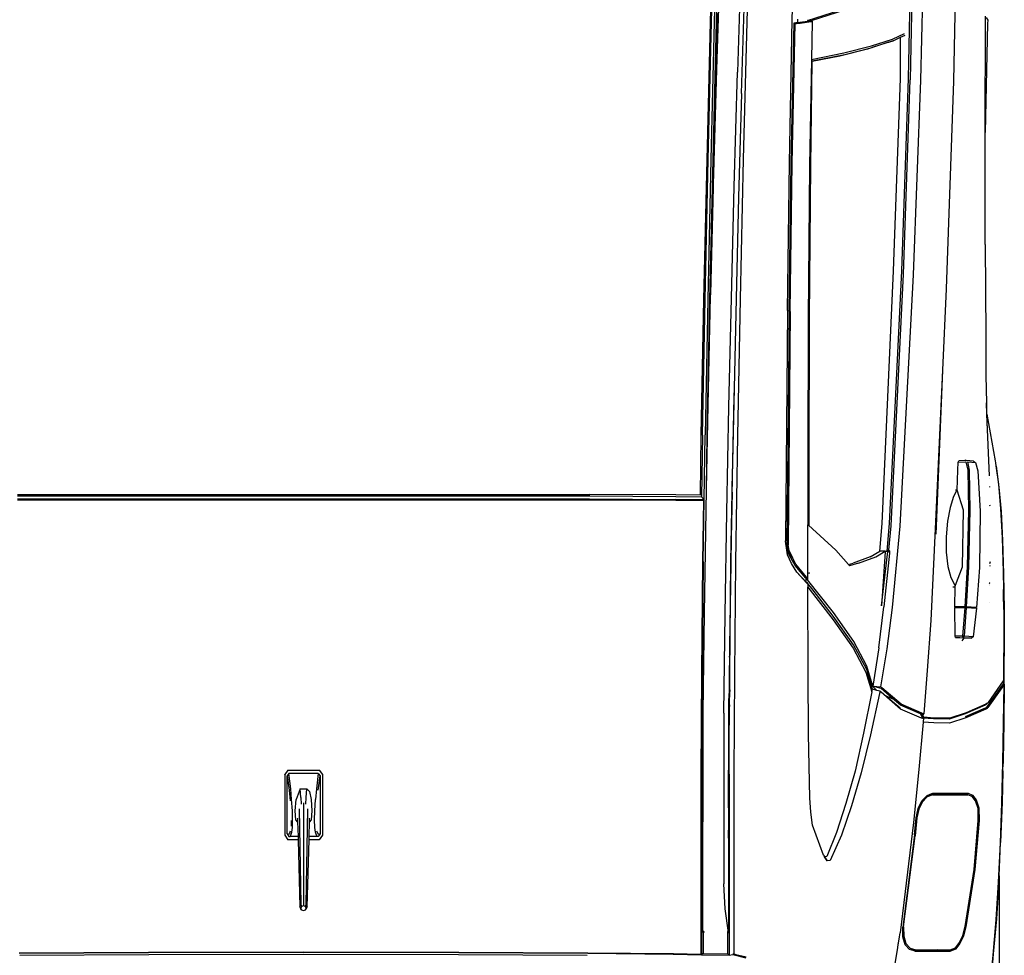
# Model space of a CAD drawing. Units: inches. Extents: x 0 to 4258, y 0 to 3769.
# Tile 9 of 30: x 3749 to 3790, y 3003 to 3042. Entities that reach past the tile are written whole.
import ezdxf

# ---------------------------------------------------------------- set-up
doc = ezdxf.new("R2010")
doc.units = ezdxf.units.IN
doc.header["$MEASUREMENT"] = 0
doc.layers.get('0').update_dxf_attribs({"color": 16})
doc.layers.add('C-PKNG-VEHI', color=8, linetype='Continuous', lineweight=18)
doc.layers.add('Edges', color=250, linetype='Continuous')

# ---------------------------------------------------------------- blocks, each defined once
blk = doc.blocks.new('Nissan Qashqai pl')
at = {"layer": 'Edges'}
for p, q in [((10.4573, 12.8093), (10.4889, 12.8119)), ((10.4613, 12.8099), (10.4926, 12.8125)), ((10.4889, 12.8119), (10.526, 12.8138)), ((10.4926, 12.8125), (10.5294, 12.8143)), ((10.526, 12.8138), (10.569, 12.8151)), ((10.5294, 12.8143), (10.5719, 12.8156)), ((10.569, 12.8151), (10.5919, 12.8155)), ((10.5719, 12.8156), (10.6176, 12.8164)), ((10.5919, 12.8155), (10.6151, 12.8159)), ((10.5981, 12.8157), (10.5919, 12.8155)), ((10.6174, 12.816), (10.5981, 12.8157)), ((10.6151, 12.8159), (10.6644, 12.8162)), ((10.6176, 12.8164), (10.6651, 12.8167)), ((10.6644, 12.8162), (10.7078, 12.8159)), ((10.6651, 12.8167), (10.666, 12.8167)), ((10.666, 12.8167), (10.677, 12.8167)), ((10.6729, 12.8157), (10.7082, 12.8156)), ((10.6809, 12.8167), (10.677, 12.8167)), ((10.7128, 12.8166), (10.6809, 12.8167)), ((10.7078, 12.8159), (10.7083, 12.8156)), ((10.7082, 12.8156), (10.7078, 12.8159)), ((10.7085, 12.8153), (10.7082, 12.8156)), ((10.7082, 12.8156), (10.7083, 12.8156)), ((10.7083, 12.8156), (10.7087, 12.8153)), ((10.7083, 12.8156), (10.7125, 12.8156)), ((10.7087, 12.8153), (10.7363, 12.7959)), ((10.7139, 12.8164), (10.7125, 12.8156)), ((10.7137, 12.8148), (10.7125, 12.8156)), ((10.7128, 12.8166), (10.7625, 12.8161)), ((10.7128, 12.8166), (10.724, 12.8166)), ((10.7137, 12.8148), (10.7138, 12.8147)), ((10.7418, 12.7947), (10.7138, 12.8147)), ((10.7139, 12.8164), (10.7148, 12.8157)), ((10.7628, 12.8158), (10.7139, 12.8164)), ((10.7148, 12.8157), (10.7429, 12.7956)), ((10.7685, 12.8161), (10.724, 12.8166)), ((10.7625, 12.8161), (10.7628, 12.8161)), ((10.7628, 12.8161), (10.8099, 12.8152)), ((10.8131, 12.8149), (10.7628, 12.8158)), ((10.7688, 12.8161), (10.7685, 12.8161)), ((10.8099, 12.8152), (10.7688, 12.8161)), ((10.8099, 12.8152), (10.8131, 12.8152)), ((10.8134, 12.8152), (10.8131, 12.8152)), ((10.8644, 12.8135), (10.8131, 12.8149)), ((10.8134, 12.8152), (10.8142, 12.8152)), ((10.8142, 12.8152), (10.8142, 12.8152)), ((10.8237, 12.8149), (10.8142, 12.8152)), ((10.8237, 12.8149), (10.864, 12.8138)), ((10.8596, 12.8138), (10.8589, 12.8138)), ((10.8642, 12.8136), (10.8596, 12.8138)), ((10.864, 12.8138), (10.8642, 12.8138)), ((10.8642, 12.8138), (10.9152, 12.812)), ((10.9158, 12.8118), (10.8644, 12.8135)), ((10.9577, 12.8101), (10.9152, 12.812)), ((10.9657, 12.8095), (10.9158, 12.8118)), ((10.9577, 12.8101), (10.9649, 12.8097)), ((10.9577, 12.8101), (11.1283, 12.8101)), ((10.3679, 12.7944), (10.4275, 12.8051)), ((10.4468, 12.7976), (10.3679, 12.7944)), ((10.4275, 12.8051), (10.4304, 12.8056)), ((10.4304, 12.8056), (10.4339, 12.8061)), ((10.4339, 12.8061), (10.4573, 12.8093)), ((10.4339, 12.8061), (10.4345, 12.8062)), ((10.4345, 12.8062), (10.4613, 12.8099)), ((10.4503, 12.7976), (10.4502, 12.7976)), ((10.4603, 12.7976), (10.4613, 12.7978)), ((10.4838, 12.7977), (10.4852, 12.7982)), ((10.5565, 12.7985), (10.5591, 12.7977)), ((10.5615, 12.7978), (10.5617, 12.7985)), ((10.583, 12.7984), (10.5834, 12.798)), ((10.5836, 12.798), (10.5831, 12.7984)), ((10.5847, 12.798), (10.5841, 12.7984)), ((10.5873, 12.7981), (10.5873, 12.7981)), ((10.6087, 12.7983), (10.6087, 12.7984)), ((10.9649, 12.8097), (11.0127, 12.8067)), ((11.0138, 12.8064), (10.9657, 12.8095)), ((11.0127, 12.8067), (11.0576, 12.8026)), ((11.059, 12.8023), (11.0138, 12.8064)), ((11.0576, 12.8026), (11.0798, 12.8008)), ((11.0768, 12.8008), (11.059, 12.8023)), ((9.8643, 12.7927), (9.8598, 12.7928)), ((9.8614, 12.7937), (9.8647, 12.7956)), ((10.0085, 12.7922), (9.8643, 12.7927)), ((9.8647, 12.7956), (9.869, 12.7954)), ((9.869, 12.7954), (10.0085, 12.7922)), ((10.0124, 12.7922), (10.0085, 12.7922)), ((10.1513, 12.7924), (10.0124, 12.7922)), ((10.1513, 12.7924), (10.2677, 12.793)), ((10.2677, 12.793), (10.3189, 12.7931)), ((10.3189, 12.7931), (10.3537, 12.7939)), ((10.3537, 12.7939), (10.3832, 12.7945)), ((10.3679, 12.7944), (10.3537, 12.7939)), ((10.4406, 12.7829), (10.4919, 12.7858)), ((10.4919, 12.7858), (10.564, 12.7851)), ((10.564, 12.7851), (10.6151, 12.7813)), ((10.7363, 12.7959), (10.7376, 12.795)), ((10.7387, 12.794), (10.7376, 12.795)), ((10.7376, 12.795), (10.7378, 12.7946)), ((10.7378, 12.7946), (10.7379, 12.7945)), ((10.7378, 12.7946), (10.7385, 12.7932)), ((10.7385, 12.7932), (10.7497, 12.7679)), ((10.7387, 12.794), (10.7396, 12.7922)), ((10.7396, 12.7922), (10.7507, 12.7669)), ((10.743, 12.7939), (10.7418, 12.7947)), ((10.7432, 12.7954), (10.7426, 12.7954)), ((10.7429, 12.7956), (10.7432, 12.7954)), ((10.7434, 12.793), (10.743, 12.7939)), ((10.7441, 12.7954), (10.7432, 12.7954)), ((10.7432, 12.7954), (10.744, 12.7948)), ((10.7437, 12.7921), (10.7434, 12.793)), ((10.7438, 12.7921), (10.7437, 12.7921)), ((10.7438, 12.7921), (10.7549, 12.7666)), ((10.744, 12.7948), (10.7448, 12.793)), ((10.7448, 12.793), (10.7559, 12.7674)), ((10.4282, 12.7775), (10.4274, 12.7679)), ((10.4282, 12.7775), (10.4299, 12.7798)), ((10.4291, 12.77), (10.4299, 12.7798)), ((10.4398, 12.7724), (10.4291, 12.77)), ((10.4299, 12.7798), (10.4406, 12.7829)), ((10.4909, 12.773), (10.4398, 12.7724)), ((10.5631, 12.7715), (10.4909, 12.773)), ((10.615, 12.7803), (10.6142, 12.7686)), ((10.6151, 12.7813), (10.615, 12.7803)), ((10.615, 12.7676), (10.6151, 12.7803)), ((10.6151, 12.7803), (10.615, 12.7803)), ((10.6151, 12.7803), (10.6151, 12.7813)), ((10.6151, 12.7685), (10.616, 12.7812)), ((10.616, 12.7812), (10.6526, 12.7768)), ((10.6526, 12.7768), (10.6518, 12.7657)), ((10.6526, 12.7768), (10.6543, 12.7749)), ((10.6537, 12.7658), (10.6543, 12.7749)), ((10.6543, 12.7749), (10.6543, 12.7656)), ((10.8523, 12.7704), (10.8546, 12.7762)), ((10.8565, 12.7757), (10.8543, 12.7702)), ((10.8546, 12.7762), (10.8607, 12.7808)), ((10.8622, 12.7801), (10.8565, 12.7757)), ((10.8607, 12.7808), (10.8708, 12.7841)), ((10.8716, 12.7832), (10.8622, 12.7801)), ((10.8708, 12.7841), (10.8869, 12.7844)), ((10.887, 12.7835), (10.8716, 12.7832)), ((10.8869, 12.7844), (10.9499, 12.7789)), ((10.9498, 12.7781), (10.887, 12.7835)), ((11.0226, 12.7668), (10.9498, 12.7781)), ((10.9499, 12.7789), (11.0229, 12.7676)), ((10.4263, 12.7665), (10.4274, 12.7674)), ((10.4274, 12.7679), (10.4274, 12.7674)), ((10.4274, 12.7674), (10.4275, 12.7586)), ((10.4291, 12.7677), (10.4398, 12.7701)), ((10.4293, 12.7579), (10.4291, 12.7677)), ((10.4398, 12.7701), (10.4909, 12.7708)), ((10.4908, 12.7648), (10.4653, 12.7564)), ((10.563, 12.7633), (10.4908, 12.7648)), ((10.4909, 12.7708), (10.563, 12.7692)), ((10.563, 12.7692), (10.6142, 12.7663)), ((10.5867, 12.7545), (10.563, 12.7633)), ((10.6142, 12.7686), (10.5631, 12.7715)), ((10.6142, 12.766), (10.6141, 12.7537)), ((10.6142, 12.7686), (10.6142, 12.7677)), ((10.6142, 12.7677), (10.615, 12.7676)), ((10.6142, 12.7677), (10.6142, 12.7663)), ((10.6142, 12.7663), (10.6142, 12.766)), ((10.6151, 12.7676), (10.615, 12.7676)), ((10.615, 12.7537), (10.6151, 12.7659)), ((10.6518, 12.7657), (10.6151, 12.7685)), ((10.6151, 12.7676), (10.6151, 12.7685)), ((10.6151, 12.7662), (10.6151, 12.7676)), ((10.6151, 12.7662), (10.6518, 12.7634)), ((10.6151, 12.7659), (10.6151, 12.7662)), ((10.6518, 12.7634), (10.6517, 12.754)), ((10.6536, 12.7639), (10.6518, 12.7657)), ((10.6518, 12.7657), (10.6518, 12.7634)), ((10.6518, 12.7634), (10.6536, 12.7639)), ((10.6543, 12.7656), (10.6535, 12.7546)), ((10.6535, 12.7546), (10.6536, 12.7639)), ((10.6536, 12.7639), (10.6537, 12.7658)), ((10.6537, 12.7658), (10.6543, 12.7656)), ((10.6578, 12.7628), (10.6543, 12.7656)), ((10.7497, 12.7679), (10.7565, 12.7473)), ((10.7507, 12.7669), (10.7575, 12.7462)), ((10.7559, 12.7674), (10.7626, 12.7467)), ((10.8523, 12.7255), (10.8523, 12.7704)), ((10.8543, 12.7702), (10.8538, 12.753)), ((10.8543, 12.7255), (10.8543, 12.7702)), ((11.0339, 12.7639), (11.0226, 12.7668)), ((11.0229, 12.7676), (11.0348, 12.7645)), ((11.0429, 12.7597), (11.0339, 12.7639)), ((11.0348, 12.7645), (11.0444, 12.7601)), ((11.0497, 12.7542), (11.0429, 12.7597)), ((11.0444, 12.7601), (11.0516, 12.7542)), ((9.8024, 12.7549), (9.9426, 12.7518)), ((9.9426, 12.7518), (10.2081, 12.7424)), ((10.4293, 12.7579), (10.4275, 12.7586)), ((10.4398, 12.7573), (10.4293, 12.7579)), ((10.4653, 12.7564), (10.4398, 12.7573)), ((10.4653, 12.7561), (10.4652, 12.7545)), ((10.4653, 12.7564), (10.4653, 12.7561)), ((10.4653, 12.7564), (10.4653, 12.7564)), ((10.4653, 12.7564), (10.4653, 12.7561)), ((10.4653, 12.7561), (10.4653, 12.7561)), ((10.4653, 12.7561), (10.4732, 12.7517)), ((10.4732, 12.7517), (10.4871, 12.7474)), ((10.4871, 12.7474), (10.5048, 12.744)), ((10.5625, 12.7446), (10.5769, 12.7484)), ((10.5769, 12.7484), (10.5863, 12.7537)), ((10.5863, 12.7537), (10.5867, 12.7545)), ((10.5885, 12.7538), (10.5867, 12.7545)), ((10.5885, 12.751), (10.5885, 12.7538)), ((10.6141, 12.7537), (10.5885, 12.7538)), ((10.6141, 12.7537), (10.615, 12.7537)), ((10.6517, 12.754), (10.615, 12.7537)), ((10.6535, 12.7546), (10.6517, 12.754)), ((10.7565, 12.7473), (10.7563, 12.7273)), ((10.8528, 12.7503), (10.8535, 12.7521)), ((10.8528, 12.742), (10.8528, 12.7503)), ((10.8535, 12.7521), (10.8538, 12.753)), ((10.8538, 12.7521), (10.8535, 12.7521)), ((10.8538, 12.753), (10.8538, 12.7521)), ((10.8538, 12.7521), (10.8538, 12.7502)), ((10.8538, 12.7502), (10.8538, 12.742)), ((11.0523, 12.7475), (11.0497, 12.7542)), ((11.0516, 12.7542), (11.0543, 12.7473)), ((11.0528, 12.73), (11.0523, 12.7475)), ((11.0523, 12.7312), (11.0523, 12.7475)), ((11.0543, 12.7473), (11.0543, 12.7035)), ((10.2081, 12.7424), (10.312, 12.7377)), ((10.312, 12.7377), (10.5214, 12.7293)), ((10.312, 12.7377), (10.5147, 12.7285)), ((10.5048, 12.744), (10.5246, 12.7423)), ((10.5246, 12.7423), (10.5445, 12.7425)), ((10.5445, 12.7425), (10.5625, 12.7446)), ((10.7575, 12.7462), (10.7572, 12.7263)), ((10.7626, 12.7467), (10.7623, 12.7269)), ((10.8528, 12.742), (10.8538, 12.742)), ((10.8528, 12.7419), (10.8528, 12.742)), ((10.8538, 12.7419), (10.8528, 12.7419)), ((10.8528, 12.7242), (10.8528, 12.7419)), ((10.8538, 12.742), (10.8538, 12.7419)), ((10.8538, 12.7214), (10.8538, 12.7419)), ((10.5147, 12.7285), (10.6318, 12.7228)), ((10.6318, 12.7228), (10.6955, 12.7184)), ((10.7563, 12.7273), (10.7553, 12.7134)), ((10.7572, 12.7263), (10.7563, 12.7126)), ((10.7623, 12.7269), (10.7615, 12.7131)), ((10.8528, 12.7242), (10.8523, 12.7255)), ((10.8538, 12.7214), (10.8528, 12.7242)), ((10.8543, 12.7255), (10.8569, 12.7184)), ((11.0523, 12.7312), (11.0528, 12.73)), ((11.0523, 12.7287), (11.0523, 12.7312)), ((11.0528, 12.7274), (11.0523, 12.7287)), ((11.0523, 12.7037), (11.0523, 12.7287)), ((11.0528, 12.7274), (11.0528, 12.73)), ((11.0528, 12.73), (11.0538, 12.7273)), ((11.0528, 12.7274), (11.0528, 12.6985)), ((11.0538, 12.7273), (11.0538, 12.7018)), ((9.9414, 12.71), (9.8143, 12.713)), ((10.19, 12.7008), (9.9414, 12.71)), ((10.6955, 12.7184), (10.7509, 12.714)), ((10.7501, 12.7114), (10.7387, 12.6849)), ((10.7507, 12.7098), (10.7397, 12.684)), ((10.7563, 12.7109), (10.7449, 12.6843)), ((10.7507, 12.7132), (10.7501, 12.7114)), ((10.7506, 12.7111), (10.7507, 12.7132)), ((10.7507, 12.7132), (10.7509, 12.714)), ((10.751, 12.7132), (10.7507, 12.7132)), ((10.7511, 12.7107), (10.7507, 12.7098)), ((10.7524, 12.7106), (10.7507, 12.7098)), ((10.7522, 12.7131), (10.7509, 12.714)), ((10.7516, 12.7131), (10.7509, 12.714)), ((10.7519, 12.7128), (10.7511, 12.7107)), ((10.7522, 12.7131), (10.7516, 12.7131)), ((10.7519, 12.7128), (10.7516, 12.7131)), ((10.7526, 12.7124), (10.7519, 12.7128)), ((10.7553, 12.7134), (10.7522, 12.7131)), ((10.7524, 12.7106), (10.7526, 12.7124)), ((10.7556, 12.7122), (10.7524, 12.7106)), ((10.7526, 12.7124), (10.7526, 12.7127)), ((10.7532, 12.712), (10.7526, 12.7124)), ((10.7556, 12.7122), (10.7532, 12.712)), ((10.7561, 12.7125), (10.7556, 12.7122)), ((10.7561, 12.7125), (10.7563, 12.7126)), ((10.7563, 12.7125), (10.7561, 12.7125)), ((10.7563, 12.7123), (10.7561, 12.7123)), ((10.7563, 12.7126), (10.7573, 12.7135)), ((10.7563, 12.7126), (10.7563, 12.7125)), ((10.7569, 12.7125), (10.7563, 12.7109)), ((10.7569, 12.7125), (10.7563, 12.7125)), ((10.7563, 12.7125), (10.7563, 12.7123)), ((10.7573, 12.7135), (10.7569, 12.7125)), ((10.7573, 12.7135), (10.7604, 12.7132)), ((10.7604, 12.7132), (10.7615, 12.7131)), ((10.7615, 12.7131), (10.8218, 12.7077)), ((10.855, 12.7181), (10.8538, 12.7214)), ((10.8622, 12.7114), (10.855, 12.7181)), ((10.8569, 12.7184), (10.8637, 12.712)), ((10.8718, 12.7068), (10.8622, 12.7114)), ((10.8637, 12.712), (10.8727, 12.7077)), ((9.8101, 12.6993), (9.9411, 12.6966)), ((9.9393, 12.6944), (9.8119, 12.697)), ((10.5113, 12.6839), (10.19, 12.7008)), ((10.8218, 12.7077), (10.8896, 12.7008)), ((10.8836, 12.7041), (10.8718, 12.7068)), ((10.8727, 12.7077), (10.8839, 12.7051)), ((10.9054, 12.702), (10.8836, 12.7041)), ((10.8839, 12.7051), (10.9067, 12.7029)), ((10.8896, 12.7008), (11.0304, 12.6838)), ((10.9054, 12.702), (11.0232, 12.6871)), ((11.0231, 12.6882), (10.9067, 12.7029)), ((11.0501, 12.6964), (11.0523, 12.7037)), ((11.0528, 12.6985), (11.052, 12.6958)), ((11.0538, 12.7018), (11.0528, 12.6985)), ((11.0543, 12.7035), (11.0538, 12.7018)), ((9.8891, 12.6741), (9.8818, 12.6891)), ((9.8867, 12.6842), (9.8838, 12.6901)), ((10.1849, 12.6857), (9.9393, 12.6944)), ((10.1894, 12.6879), (9.9411, 12.6966)), ((10.5079, 12.6703), (10.1849, 12.6857)), ((10.5109, 12.6721), (10.1894, 12.6879)), ((10.7387, 12.6849), (10.7177, 12.6604)), ((10.7449, 12.6843), (10.7232, 12.6594)), ((11.0231, 12.6882), (11.035, 12.6883)), ((11.0358, 12.6872), (11.0232, 12.6871)), ((11.035, 12.6883), (11.0443, 12.6911)), ((11.0458, 12.6903), (11.0358, 12.6872)), ((11.0443, 12.6911), (11.0501, 12.6964)), ((11.052, 12.6958), (11.0458, 12.6903)), ((9.9393, 12.684), (9.8867, 12.6842)), ((9.8911, 12.675), (9.8867, 12.6842)), ((9.8978, 12.6472), (9.8891, 12.6741)), ((9.8911, 12.6749), (9.8911, 12.675)), ((9.8931, 12.6691), (9.8911, 12.6749)), ((9.8911, 12.6749), (9.8998, 12.6481)), ((10.1849, 12.6754), (9.9393, 12.684)), ((10.5079, 12.6607), (10.1849, 12.6754)), ((10.5417, 12.6693), (10.5109, 12.6721)), ((10.6152, 12.674), (10.5113, 12.6839)), ((10.6678, 12.6672), (10.6152, 12.674)), ((10.7334, 12.6766), (10.7186, 12.6593)), ((10.7438, 12.6836), (10.7265, 12.6635)), ((10.7265, 12.6635), (10.7316, 12.6741)), ((10.7397, 12.684), (10.7334, 12.6766)), ((11.0357, 12.6829), (11.0304, 12.6838)), ((11.0491, 12.6807), (11.0357, 12.6829)), ((11.0449, 12.6812), (11.0448, 12.6812)), ((11.0492, 12.6807), (11.0491, 12.6807)), ((11.1336, 12.667), (11.0492, 12.6807)), ((9.8931, 12.669), (9.8931, 12.6691)), ((9.8931, 12.669), (9.9018, 12.6421)), ((10.543, 12.6671), (10.5079, 12.6703)), ((10.543, 12.6576), (10.5079, 12.6607)), ((10.5417, 12.6693), (10.5427, 12.6702)), ((10.5417, 12.6693), (10.543, 12.6671)), ((10.5436, 12.6687), (10.5427, 12.6702)), ((10.5427, 12.6702), (10.5458, 12.67)), ((10.544, 12.6678), (10.543, 12.6671)), ((10.543, 12.6646), (10.543, 12.6671)), ((10.543, 12.6646), (10.543, 12.6576)), ((10.5439, 12.6646), (10.543, 12.6646)), ((10.5502, 12.6526), (10.543, 12.6646)), ((10.544, 12.6678), (10.5436, 12.6687)), ((10.5439, 12.6646), (10.613, 12.6601)), ((10.547, 12.6674), (10.544, 12.6678)), ((10.5458, 12.67), (10.6144, 12.6629)), ((10.613, 12.6601), (10.547, 12.6674)), ((10.6664, 12.6566), (10.6144, 12.6629)), ((10.7137, 12.6595), (10.6678, 12.6672)), ((10.7165, 12.6591), (10.7137, 12.6595)), ((10.7186, 12.6593), (10.7155, 12.649)), ((10.7177, 12.6604), (10.7165, 12.6591)), ((10.7232, 12.6594), (10.7221, 12.6581)), ((10.7265, 12.6635), (10.7224, 12.6587)), ((9.9066, 12.6119), (9.8978, 12.6472)), ((9.9086, 12.6129), (9.8998, 12.6481)), ((10.5502, 12.6456), (10.543, 12.6576)), ((10.5584, 12.6306), (10.5502, 12.6526)), ((10.6664, 12.6566), (10.7155, 12.649)), ((10.7155, 12.649), (10.69, 12.6414)), ((10.7155, 12.6473), (10.6943, 12.641)), ((10.6976, 12.6401), (10.7228, 12.6477)), ((10.7155, 12.649), (10.7165, 12.6591)), ((10.7209, 12.654), (10.7155, 12.6485)), ((10.7155, 12.649), (10.7155, 12.6485)), ((10.7155, 12.6485), (10.7155, 12.6473)), ((10.7192, 12.6484), (10.7155, 12.6473)), ((10.7209, 12.654), (10.7192, 12.6484)), ((10.7228, 12.6477), (10.7192, 12.6484)), ((10.7221, 12.6581), (10.7209, 12.654)), ((10.7221, 12.6581), (10.7224, 12.6587)), ((10.7221, 12.6581), (10.7247, 12.6575)), ((10.7228, 12.6477), (10.7754, 12.637)), ((10.7247, 12.6575), (10.7776, 12.646)), ((9.9018, 12.6421), (9.9106, 12.6068)), ((10.5502, 12.6456), (10.5584, 12.6236)), ((10.69, 12.6414), (10.6583, 12.6245)), ((10.6943, 12.641), (10.6627, 12.6241)), ((10.6671, 12.6238), (10.6976, 12.6401)), ((10.7754, 12.637), (10.8239, 12.6261)), ((10.7776, 12.646), (10.8264, 12.6341)), ((10.8264, 12.6341), (10.8682, 12.6216)), ((10.5584, 12.6306), (10.5617, 12.619)), ((10.56, 12.6176), (10.5584, 12.6236)), ((10.6583, 12.6245), (10.6215, 12.5986)), ((10.6627, 12.6241), (10.6261, 12.5984)), ((10.6306, 12.5982), (10.6671, 12.6238)), ((10.8239, 12.6261), (10.8653, 12.6144)), ((10.8682, 12.6216), (10.9059, 12.6087)), ((9.8652, 12.5704), (9.8516, 12.6129)), ((9.9149, 12.5705), (9.9066, 12.6119)), ((9.9169, 12.5714), (9.9086, 12.6129)), ((10.5419, 12.6018), (10.56, 12.6176)), ((10.56, 12.6176), (10.5617, 12.619)), ((10.8653, 12.6144), (10.9026, 12.6025)), ((9.8652, 12.5654), (9.8516, 12.6079)), ((9.9106, 12.6068), (9.9177, 12.5714)), ((10.51, 12.5666), (10.5419, 12.6018)), ((10.6215, 12.5986), (10.5796, 12.5655)), ((10.5892, 12.5659), (10.6306, 12.5982)), ((10.6261, 12.5984), (10.593, 12.5726)), ((10.9026, 12.6025), (10.933, 12.5901)), ((10.9059, 12.6087), (10.9384, 12.5945)), ((10.9316, 12.586), (10.8932, 12.572)), ((10.9316, 12.586), (10.9334, 12.5872)), ((10.932, 12.5862), (10.9316, 12.586)), ((10.9335, 12.5871), (10.932, 12.5862)), ((10.933, 12.5901), (10.9334, 12.5872)), ((10.9334, 12.5872), (10.9386, 12.5905)), ((10.9334, 12.5872), (10.9335, 12.5871)), ((10.9386, 12.5905), (10.9335, 12.5871)), ((10.9384, 12.5945), (10.9386, 12.5905)), ((9.8652, 12.5706), (9.8664, 12.5714)), ((9.8665, 12.5695), (9.8664, 12.5714)), ((9.8664, 12.5714), (9.9149, 12.5705)), ((9.9177, 12.5714), (9.9169, 12.5714)), ((10.0501, 12.5695), (9.9177, 12.5714)), ((10.593, 12.5726), (10.584, 12.5655)), ((10.8932, 12.572), (10.8766, 12.5697)), ((9.8652, 12.5706), (9.8665, 12.5695)), ((9.8652, 12.5704), (9.8652, 12.5706)), ((9.8652, 12.5704), (9.8652, 12.5704)), ((9.8652, 12.5704), (9.8652, 12.5654)), ((9.8655, 12.5687), (9.8652, 12.5704)), ((9.8675, 12.5555), (9.8655, 12.5687)), ((9.8686, 12.5562), (9.8665, 12.5695)), ((9.9149, 12.5705), (10.0505, 12.5681)), ((10.2453, 12.568), (10.0501, 12.5695)), ((10.0505, 12.5681), (10.2453, 12.5664)), ((10.4292, 12.5674), (10.2453, 12.568)), ((10.2453, 12.5664), (10.4289, 12.5658)), ((10.4289, 12.5658), (10.5092, 12.5658)), ((10.5099, 12.5674), (10.4292, 12.5674)), ((10.5099, 12.5674), (10.5092, 12.5658)), ((10.5092, 12.5658), (10.5094, 12.5658)), ((10.5094, 12.5658), (10.51, 12.5666)), ((10.5783, 12.5659), (10.5094, 12.5658)), ((10.51, 12.5666), (10.5099, 12.5674)), ((10.5764, 12.5642), (10.5598, 12.5507)), ((10.5776, 12.5633), (10.5612, 12.5498)), ((10.5834, 12.5641), (10.57, 12.5517)), ((10.57, 12.5517), (10.5821, 12.5633)), ((10.5709, 12.5675), (10.5705, 12.5671)), ((10.5719, 12.5682), (10.5709, 12.5675)), ((10.5783, 12.5659), (10.5764, 12.5642)), ((10.5776, 12.5633), (10.5783, 12.5659)), ((10.5796, 12.5655), (10.5776, 12.5633)), ((10.5796, 12.5655), (10.5783, 12.5659)), ((10.5796, 12.562), (10.5796, 12.5655)), ((10.5838, 12.5653), (10.5821, 12.5633)), ((10.584, 12.5647), (10.5834, 12.5641)), ((10.584, 12.5655), (10.5838, 12.5653)), ((10.584, 12.5655), (10.5841, 12.5655)), ((10.584, 12.5654), (10.584, 12.5655)), ((10.5847, 12.5655), (10.584, 12.5647)), ((10.584, 12.5647), (10.584, 12.5654)), ((10.5851, 12.5659), (10.5841, 12.5655)), ((10.5841, 12.5655), (10.5847, 12.5655)), ((10.5851, 12.5659), (10.5847, 12.5655)), ((10.5851, 12.5659), (10.5892, 12.5659)), ((10.6988, 12.5662), (10.5892, 12.5659)), ((10.7769, 12.5667), (10.6988, 12.5662)), ((10.858, 12.5683), (10.7769, 12.5667)), ((10.8766, 12.5697), (10.858, 12.5683)), ((9.8644, 12.5459), (9.696, 12.551)), ((9.8643, 12.5532), (9.8637, 12.5532)), ((9.8677, 12.5531), (9.8643, 12.5532)), ((9.8677, 12.5531), (9.8675, 12.5555)), ((9.8678, 12.5507), (9.8677, 12.5531)), ((9.8681, 12.5482), (9.8678, 12.5507)), ((9.8681, 12.5482), (9.869, 12.5496)), ((10.0476, 12.5445), (9.8681, 12.5482)), ((9.8689, 12.5515), (9.8686, 12.5562)), ((9.869, 12.5496), (9.8689, 12.5515)), ((10.0477, 12.5459), (9.869, 12.5496)), ((10.5522, 12.5465), (10.5422, 12.542)), ((10.5546, 12.546), (10.5495, 12.5438)), ((10.5598, 12.5507), (10.5522, 12.5465)), ((10.5583, 12.5481), (10.5546, 12.546)), ((10.5551, 12.5457), (10.5583, 12.5481)), ((10.5612, 12.5498), (10.5583, 12.5481)), ((10.57, 12.5517), (10.5589, 12.5451)), ((10.0472, 12.5423), (9.8644, 12.5459)), ((10.2357, 12.5398), (10.0472, 12.5423)), ((10.2367, 12.5419), (10.0476, 12.5445)), ((10.2369, 12.5433), (10.0477, 12.5459)), ((10.2357, 12.5398), (10.53, 12.5373)), ((10.2367, 12.5419), (10.5351, 12.5392)), ((10.2369, 12.5433), (10.5348, 12.5406)), ((10.4153, 12.5384), (10.4176, 12.5384)), ((10.4176, 12.5384), (10.4181, 12.5384)), ((10.4181, 12.5384), (10.4552, 12.538)), ((10.4181, 12.5384), (10.4181, 12.5384)), ((10.4778, 12.5378), (10.53, 12.5373)), ((10.5301, 12.5373), (10.53, 12.5373)), ((10.5335, 12.5378), (10.5301, 12.5373)), ((10.5419, 12.5391), (10.5335, 12.5378)), ((10.5422, 12.542), (10.5348, 12.5406)), ((10.5418, 12.5405), (10.5351, 12.5392)), ((10.5424, 12.5406), (10.5418, 12.5405)), ((10.5419, 12.5391), (10.5463, 12.541)), ((10.5479, 12.54), (10.5419, 12.5391)), ((10.5495, 12.5438), (10.5424, 12.5406)), ((10.5463, 12.541), (10.5551, 12.5457)), ((10.5589, 12.5451), (10.5479, 12.54)), ((9.9583, 12.4812), (9.651, 12.4906)), ((9.6514, 12.4849), (9.9312, 12.4761)), ((9.7029, 12.4926), (9.8673, 12.4878)), ((9.8673, 12.4878), (10.0423, 12.4835)), ((10.0423, 12.4835), (10.2211, 12.4795)), ((11.0581, 12.4738), (11.0614, 12.4872)), ((11.0582, 12.47), (11.0624, 12.4866)), ((10.0776, 12.4719), (9.9312, 12.4761)), ((9.9583, 12.4812), (10.091, 12.4775)), ((10.2201, 12.4683), (10.0776, 12.4719)), ((10.091, 12.4775), (10.2202, 12.4743)), ((10.2202, 12.4743), (10.2203, 12.4743)), ((10.2203, 12.4743), (10.3353, 12.4717)), ((10.2211, 12.4795), (10.3955, 12.4762)), ((10.3353, 12.4717), (10.4477, 12.4694)), ((10.3353, 12.4717), (10.346, 12.4714)), ((10.346, 12.4714), (10.4477, 12.4694)), ((10.3955, 12.4762), (10.5572, 12.4737)), ((10.5572, 12.4737), (10.7004, 12.4722)), ((10.7004, 12.4722), (10.8279, 12.4715)), ((10.8279, 12.4715), (11.0544, 12.4714)), ((11.0544, 12.4714), (11.0575, 12.4714)), ((11.0575, 12.4714), (11.0581, 12.4738)), ((11.0575, 12.4714), (11.0582, 12.47)), ((9.6472, 12.4581), (9.9278, 12.4492)), ((10.3586, 12.4651), (10.2201, 12.4683)), ((10.4931, 12.4624), (10.3586, 12.4651)), ((10.4477, 12.4694), (10.4538, 12.4693)), ((10.4538, 12.4693), (10.4681, 12.469)), ((10.4676, 12.4691), (10.4538, 12.4693)), ((10.5566, 12.4677), (10.4676, 12.4691)), ((10.4676, 12.4691), (10.546, 12.4677)), ((10.4681, 12.469), (10.5866, 12.467)), ((10.6237, 12.4603), (10.4931, 12.4624)), ((10.546, 12.4677), (10.546, 12.4678)), ((10.546, 12.4677), (10.5576, 12.4675)), ((10.7, 12.4662), (10.5566, 12.4677)), ((10.5576, 12.4675), (10.6649, 12.4659)), ((10.5866, 12.467), (10.6649, 12.4659)), ((10.7502, 12.4586), (10.6237, 12.4603)), ((10.6649, 12.4659), (10.6786, 12.4658)), ((10.6649, 12.4659), (10.6772, 12.4657)), ((10.6786, 12.4657), (10.6772, 12.4657)), ((10.6786, 12.4658), (10.6786, 12.4662)), ((10.6786, 12.4657), (10.6786, 12.4658)), ((10.6786, 12.4658), (10.6801, 12.4657)), ((10.6786, 12.4657), (10.6801, 12.4657)), ((10.6801, 12.4662), (10.6801, 12.4657)), ((10.6801, 12.4657), (10.6801, 12.4657)), ((10.6801, 12.4657), (10.6811, 12.4657)), ((10.6801, 12.4657), (10.6811, 12.4657)), ((10.6811, 12.4662), (10.6811, 12.4657)), ((10.6811, 12.4657), (10.6811, 12.4657)), ((10.6811, 12.4657), (10.6966, 12.4654)), ((10.6811, 12.4657), (10.6991, 12.4655)), ((10.6811, 12.4657), (10.6991, 12.4655)), ((10.6966, 12.4654), (10.7144, 12.4653)), ((10.6991, 12.4655), (10.7144, 12.4653)), ((10.7201, 12.4661), (10.7, 12.4662)), ((10.7144, 12.4653), (10.7239, 12.4653)), ((10.7201, 12.4661), (10.7306, 12.4653)), ((10.7395, 12.4659), (10.7201, 12.4661)), ((10.7239, 12.4653), (10.7248, 12.4653)), ((10.7306, 12.4653), (10.7248, 12.4653)), ((10.7311, 12.4652), (10.7306, 12.4653)), ((10.7495, 12.4652), (10.7311, 12.4652)), ((10.7311, 12.4652), (10.7502, 12.4651)), ((10.7395, 12.4659), (10.7495, 12.4652)), ((10.7923, 12.4656), (10.7395, 12.4659)), ((10.8179, 12.4648), (10.7495, 12.4652)), ((10.7502, 12.4651), (10.7504, 12.4651)), ((10.7502, 12.4586), (10.968, 12.4585)), ((10.7504, 12.4651), (10.7808, 12.4649)), ((10.7808, 12.4649), (10.8179, 12.4648)), ((10.7923, 12.4652), (10.7923, 12.4656)), ((10.7933, 12.4656), (10.7923, 12.4656)), ((10.7933, 12.4652), (10.7933, 12.4656)), ((10.804, 12.4656), (10.7933, 12.4656)), ((10.804, 12.4653), (10.804, 12.4656)), ((10.8075, 12.4655), (10.804, 12.4656)), ((10.8075, 12.4655), (10.8075, 12.4653)), ((10.811, 12.4655), (10.8075, 12.4655)), ((10.811, 12.4655), (10.811, 12.4653)), ((10.8145, 12.4655), (10.811, 12.4655)), ((10.8145, 12.4653), (10.8145, 12.4655)), ((10.8279, 12.4654), (10.8145, 12.4655)), ((10.8277, 12.4647), (10.8179, 12.4648)), ((10.8711, 12.4646), (10.8277, 12.4647)), ((10.8279, 12.4654), (11.0592, 12.4653)), ((10.8711, 12.4646), (10.8824, 12.4646)), ((10.8824, 12.4646), (10.8825, 12.4646)), ((10.8825, 12.4646), (10.8884, 12.4646)), ((10.8884, 12.4646), (10.8923, 12.4646)), ((10.8923, 12.4646), (10.8996, 12.4646)), ((10.9097, 12.4646), (10.8996, 12.4646)), ((10.9097, 12.4646), (10.9399, 12.4646)), ((10.9399, 12.4646), (10.9491, 12.4645)), ((10.9491, 12.4645), (11.0301, 12.4645)), ((11, 12.4605), (10.968, 12.4585)), ((11.0301, 12.4645), (11, 12.4605)), ((11.0301, 12.4637), (11.0287, 12.4637)), ((11.03, 12.4635), (11.0301, 12.4637)), ((11.0301, 12.4642), (11.0301, 12.4645)), ((11.0574, 12.4637), (11.0301, 12.4637)), ((11.0568, 12.4323), (11.0574, 12.4637)), ((11.0574, 12.4637), (11.0592, 12.4653)), ((11.0592, 12.4653), (11.0582, 12.47)), ((11.0585, 12.43), (11.0592, 12.4653)), ((9.701, 12.4459), (9.8673, 12.441)), ((9.8673, 12.443), (9.7011, 12.4478)), ((9.7014, 12.4536), (9.8673, 12.4488)), ((9.7014, 12.4513), (9.8673, 12.4464)), ((9.9794, 12.4475), (9.8565, 12.451)), ((9.8673, 12.4488), (10.0429, 12.4444)), ((9.8673, 12.4464), (10.0429, 12.4421)), ((9.9278, 12.4492), (10.0747, 12.445)), ((10.0998, 12.4443), (9.9794, 12.4475)), ((10.043, 12.4387), (9.8673, 12.443)), ((9.8673, 12.441), (10.0431, 12.4367)), ((10.0429, 12.4444), (10.2216, 12.4404)), ((10.0429, 12.4421), (10.2215, 12.4381)), ((10.2218, 12.4347), (10.043, 12.4387)), ((10.0431, 12.4367), (10.2218, 12.4327)), ((10.0747, 12.445), (10.078, 12.4449)), ((10.078, 12.4449), (10.2146, 12.4414)), ((10.2146, 12.4414), (10.0998, 12.4443)), ((10.2146, 12.4414), (10.2175, 12.4413)), ((10.2175, 12.4413), (10.3564, 12.4382)), ((10.2215, 12.4381), (10.3945, 12.4348)), ((10.2216, 12.4404), (10.3947, 12.4371)), ((10.3947, 12.4314), (10.2218, 12.4347)), ((10.3564, 12.4382), (10.4638, 12.436)), ((10.4773, 12.4335), (10.3945, 12.4348)), ((10.3947, 12.4371), (10.4638, 12.436)), ((10.4638, 12.436), (10.4914, 12.4355)), ((10.4735, 12.4301), (10.4773, 12.4335)), ((10.4773, 12.4335), (10.4773, 12.4296)), ((10.4785, 12.433), (10.4773, 12.4335)), ((10.5561, 12.4323), (10.4773, 12.4335)), ((10.4781, 12.3972), (10.4785, 12.433)), ((10.5563, 12.4318), (10.4785, 12.433)), ((10.4914, 12.4355), (10.6223, 12.4333)), ((10.6223, 12.4333), (10.7493, 12.4316)), ((11.0295, 12.4341), (11.0295, 12.4343)), ((10.2218, 12.4327), (10.3947, 12.4294)), ((10.3947, 12.4314), (10.4735, 12.4301)), ((10.3947, 12.4294), (10.4715, 12.4282)), ((10.4715, 12.4282), (10.4711, 12.3973)), ((10.4731, 12.3973), (10.4735, 12.4301)), ((10.4773, 12.4296), (10.4769, 12.3968)), ((10.5561, 12.4323), (10.6996, 12.4308)), ((10.6999, 12.4304), (10.5563, 12.4318)), ((10.6996, 12.4308), (10.7722, 12.4304)), ((10.827, 12.4297), (10.6999, 12.4304)), ((10.7493, 12.4316), (11.0294, 12.4315)), ((10.7722, 12.4304), (10.7722, 12.4302)), ((10.7722, 12.4304), (10.7889, 12.4303)), ((10.7889, 12.4302), (10.7889, 12.4303)), ((10.7889, 12.4303), (10.7923, 12.4303)), ((10.7923, 12.4302), (10.7923, 12.4303)), ((10.7923, 12.4303), (10.7933, 12.4303)), ((10.7933, 12.4302), (10.7933, 12.4303)), ((10.7933, 12.4303), (10.8267, 12.4301)), ((10.8267, 12.4301), (11.0585, 12.43)), ((10.9133, 12.4296), (10.827, 12.4297)), ((10.9133, 12.4296), (10.9133, 12.4298)), ((10.9137, 12.4296), (10.9133, 12.4296)), ((10.9137, 12.4296), (10.9138, 12.4298)), ((10.9715, 12.4296), (10.9137, 12.4296)), ((10.9715, 12.4299), (10.9715, 12.4296)), ((11.0579, 12.4296), (10.9715, 12.4296)), ((11.0281, 12.4323), (11.0568, 12.4323)), ((11.0294, 12.4315), (11.0294, 12.4316)), ((11.0568, 12.4323), (11.0585, 12.43)), ((11.0572, 12.3942), (11.0579, 12.4296)), ((11.0579, 12.3938), (11.0585, 12.43)), ((11.0579, 12.4296), (11.0585, 12.43)), ((10.4711, 12.3973), (10.4706, 12.2875)), ((10.4726, 12.2875), (10.4731, 12.3973)), ((10.4764, 12.2872), (10.4769, 12.3968)), ((10.4776, 12.2874), (10.4781, 12.3972)), ((11.056, 12.2851), (11.0572, 12.3942)), ((11.0566, 12.2849), (11.0579, 12.3938)), ((10.4706, 11.5566), (10.4706, 12.2875)), ((10.4726, 11.5567), (10.4726, 12.2875)), ((10.4764, 11.5569), (10.4764, 12.2872)), ((10.4776, 11.5567), (10.4776, 12.2874)), ((11.0551, 12.1203), (11.056, 12.2851)), ((11.0557, 12.1202), (11.0566, 12.2849)), ((11.0595, 12.2842), (11.0586, 12.1198)), ((11.0547, 11.9221), (11.0551, 12.1203)), ((11.0554, 11.9221), (11.0557, 12.1202)), ((11.0586, 12.1198), (11.0583, 11.9221)), ((10.8228, 11.9421), (10.8283, 11.9461)), ((10.827, 11.9408), (10.8301, 11.9431)), ((10.8279, 11.9461), (10.8283, 11.9461)), ((10.8283, 11.9461), (10.906, 11.9461)), ((10.8483, 11.9406), (10.8301, 11.9431)), ((10.8301, 11.9431), (10.9043, 11.9431)), ((10.9043, 11.9431), (10.9074, 11.9408)), ((10.9043, 11.9431), (10.905, 11.9414)), ((10.906, 11.9461), (10.9116, 11.9421)), ((10.8228, 11.9421), (10.8224, 11.9421)), ((10.8228, 11.9021), (10.8228, 11.9421)), ((10.827, 11.9408), (10.827, 11.9033)), ((10.827, 11.9408), (10.8467, 11.9386)), ((10.8467, 11.9386), (10.8603, 11.9373)), ((10.8501, 11.9295), (10.8603, 11.9316)), ((10.8746, 11.9363), (10.8603, 11.9373)), ((10.8603, 11.9316), (10.8746, 11.9327)), ((10.8861, 11.9361), (10.8746, 11.9363)), ((10.8746, 11.9327), (10.8861, 11.9319)), ((10.8959, 11.9365), (10.8861, 11.9361)), ((10.8861, 11.9319), (10.889, 11.9296)), ((10.9021, 11.9372), (10.8959, 11.9365)), ((10.9035, 11.9403), (10.9008, 11.9391)), ((10.9057, 11.9384), (10.9021, 11.9372)), ((10.905, 11.9414), (10.9035, 11.9403)), ((10.9074, 11.9393), (10.9057, 11.9384)), ((10.9074, 11.9408), (10.9074, 11.9393)), ((10.9074, 11.9393), (10.9074, 11.9291)), ((10.9116, 11.9421), (10.9116, 11.929)), ((10.8467, 11.9263), (10.8501, 11.9295)), ((10.8467, 11.9178), (10.8467, 11.9263)), ((10.8579, 11.9255), (10.8467, 11.9263)), ((10.8579, 11.9187), (10.8467, 11.9178)), ((10.8467, 11.9178), (10.8603, 11.9126)), ((10.8662, 11.925), (10.8579, 11.9255)), ((10.8579, 11.9187), (10.8662, 11.9191)), ((10.8647, 11.9221), (10.996, 11.9221)), ((10.9946, 11.9254), (10.872, 11.9276)), ((10.8723, 11.9165), (10.9946, 11.9187)), ((10.889, 11.9296), (10.884, 11.9298)), ((10.9074, 11.9291), (10.889, 11.9296)), ((10.9116, 11.929), (10.9074, 11.9291)), ((10.9973, 11.9268), (10.9116, 11.929)), ((10.9969, 11.9247), (10.9946, 11.9254)), ((10.9946, 11.9187), (10.9969, 11.9195)), ((10.9969, 11.9247), (10.996, 11.9221)), ((10.996, 11.9221), (10.9969, 11.9195)), ((10.999, 11.9258), (10.9969, 11.9247)), ((10.9969, 11.9195), (10.999, 11.9184)), ((10.9973, 11.9268), (11.0001, 11.9254)), ((10.999, 11.9258), (10.9973, 11.9268)), ((11.0001, 11.9187), (10.9973, 11.9173)), ((10.9973, 11.9173), (10.999, 11.9184)), ((11.0012, 11.9247), (10.999, 11.9258)), ((10.999, 11.9184), (10.9996, 11.9187)), ((10.9996, 11.9187), (11.0012, 11.9195)), ((11.0001, 11.9187), (10.9996, 11.9187)), ((11.0012, 11.9247), (11.0001, 11.9254)), ((11.0012, 11.9195), (11.0001, 11.9187)), ((11.002, 11.9221), (11.0012, 11.9247)), ((11.0012, 11.9195), (11.002, 11.9221)), ((11.0551, 11.7239), (11.0547, 11.9221)), ((11.0557, 11.724), (11.0554, 11.9221)), ((11.0583, 11.9221), (11.0586, 11.7244)), ((10.8467, 11.9056), (10.827, 11.9033)), ((10.8603, 11.9068), (10.8467, 11.9056)), ((10.8483, 11.9036), (10.8619, 11.905)), ((10.8746, 11.9115), (10.8603, 11.9126)), ((10.8746, 11.9078), (10.8603, 11.9068)), ((10.8861, 11.9122), (10.8746, 11.9115)), ((10.8861, 11.908), (10.8746, 11.9078)), ((10.884, 11.9144), (10.889, 11.9145)), ((10.889, 11.9145), (10.8861, 11.9122)), ((10.8959, 11.9077), (10.8861, 11.908)), ((10.8871, 11.9063), (10.8944, 11.906)), ((10.889, 11.9145), (10.9074, 11.915)), ((10.9021, 11.9069), (10.8959, 11.9077)), ((10.9008, 11.905), (10.9035, 11.9039)), ((10.9057, 11.9058), (10.9021, 11.9069)), ((10.9074, 11.9049), (10.9057, 11.9058)), ((10.9074, 11.915), (10.9116, 11.9151)), ((10.9074, 11.915), (10.9074, 11.9049)), ((10.9074, 11.9033), (10.9074, 11.9049)), ((10.9116, 11.9151), (10.9973, 11.9173)), ((10.9116, 11.9151), (10.9116, 11.9021)), ((10.8224, 11.9021), (10.8228, 11.9021)), ((10.8228, 11.9021), (10.8283, 11.8981)), ((10.827, 11.9033), (10.8301, 11.9011)), ((10.8283, 11.8981), (10.8279, 11.8981)), ((10.8283, 11.8981), (10.906, 11.8981)), ((10.8301, 11.9011), (10.8483, 11.9036)), ((10.9043, 11.9011), (10.8301, 11.9011)), ((10.9035, 11.9039), (10.905, 11.9028)), ((10.9043, 11.9011), (10.9074, 11.9033)), ((10.905, 11.9028), (10.9043, 11.9011)), ((10.906, 11.8981), (10.9116, 11.9021)), ((10.9074, 11.9033), (10.9074, 11.9048)), ((11.056, 11.559), (11.0551, 11.7239)), ((11.0566, 11.5593), (11.0557, 11.724)), ((11.0586, 11.7244), (11.0595, 11.5599))]:
    blk.add_line(p, q, dxfattribs=at)
blk = doc.blocks.new('car')
blk.add_blockref('Nissan Qashqai pl', (-9.7433, -11.9151))

msp = doc.modelspace()

# ---------------------------------------------------------------- block references
at = {"layer": 'C-PKNG-VEHI', "xscale": 32.66500240257601, "yscale": 32.66500240257601, "zscale": 32.66500240257601, "rotation": 270}
msp.add_blockref('car', (3760.419, 3045.57), dxfattribs=at)

doc.saveas('drawing.dxf')
